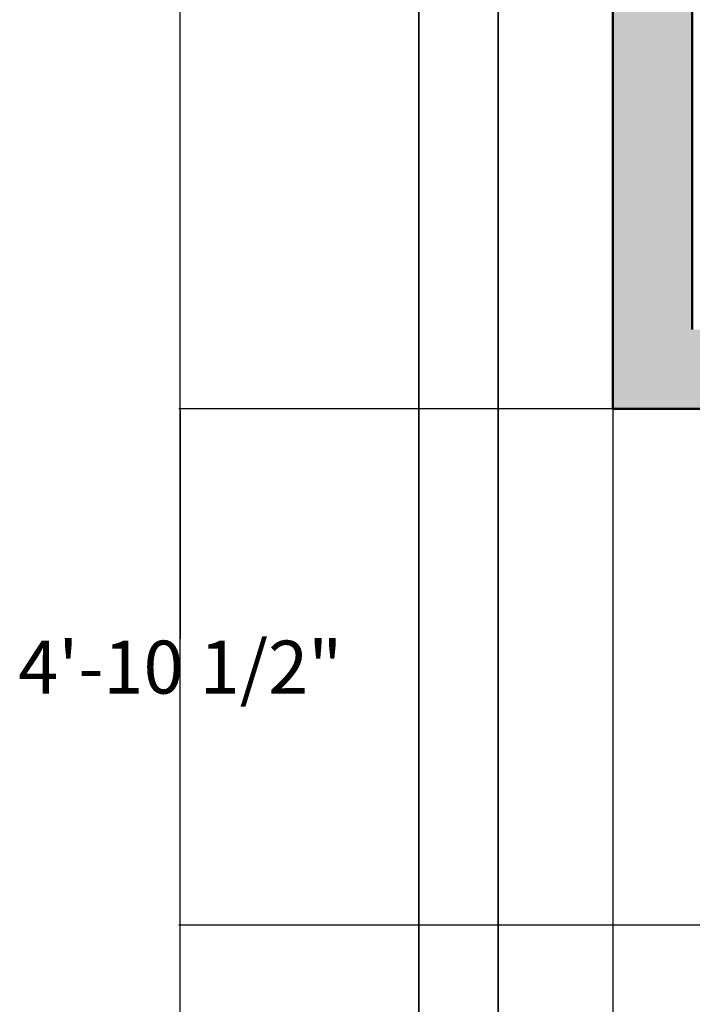
# Model space of a CAD drawing. Units: inches. Extents: x 3398 to 3816, y 15195 to 15771.
# Tile 2 of 10: x 3398 to 3474, y 15306 to 15418. Entities that reach past the tile are written whole.
import ezdxf

# ---------------------------------------------------------------- set-up
doc = ezdxf.new("R2010")
doc.units = ezdxf.units.IN
doc.header["$MEASUREMENT"] = 0
for name, color, linetype, lineweight in [('A-ANNO-DIMS', 2, 'Continuous', 18), ('A-WALL', 7, 'Continuous', 50), ('A-WALL-PATT', 252, 'Continuous', 13), ('C-PROP', 7, 'Continuous', 35)]:
    doc.layers.add(name, color=color, linetype=linetype, lineweight=lineweight)
doc.styles.get("Standard").update_dxf_attribs({"font": 'arial.ttf'})
doc.dimstyles.get("Standard").update_dxf_attribs({"dimtxt": 6, "dimasz": 0.18, "dimexe": 0.18, "dimexo": 0.0625, "dimgap": 0.09, "dimtad": 0, "dimtih": 1, "dimtoh": 1, "dimdec": 1, "dimzin": 0, "dimdsep": 46, "dimlunit": 3, "dimtxsty": 'Standard', "dimcen": 0.09, "dimadec": 0, "dimazin": 0, "dimtfac": 1, "dimtdec": 1, "dimtofl": 0, "dimtmove": 0, "dimatfit": 3, "dimfxl": 1, "dimtolj": 1, "dimtzin": 0, "dimarcsym": 0})

# ---------------------------------------------------------------- blocks, each defined once
blk = doc.blocks.new('*D38')
at = {"layer": 'A-ANNO-DIMS', "color": 0, "lineweight": -2, "transparency": 16777216}
for p, q in [((3465.13, 15730.52), (3415.96, 15730.52)), ((3416.14, 15730.34), (3416.14, 15483.67)), ((3416.14, 15230.7), (3416.14, 15477.37)), ((3465.74, 15230.52), (3415.96, 15230.52))]:
    blk.add_line(p, q, dxfattribs=at)
at = {"layer": 'A-ANNO-DIMS', "color": 0, "transparency": 16777216}
for points in [[(3416.11, 15730.34), (3416.17, 15730.34), (3416.14, 15730.52)], [(3416.11, 15230.7), (3416.17, 15230.7), (3416.14, 15230.52)]]:
    blk.add_solid(points, dxfattribs=at)
at = {"layer": 'Defpoints', "color": 0, "transparency": 16777216}
for p in [(3416.14, 15730.52), (3465.19, 15730.52), (3465.8, 15230.52)]:
    blk.add_point(p, dxfattribs=at)
at = {"layer": 'A-ANNO-DIMS', "color": 0, "transparency": 16777216, "insert": (3416.14, 15480.52), "char_height": 6, "attachment_point": 5}
blk.add_mtext('\\A1;41\'-8"', dxfattribs=at)
blk = doc.blocks.new('*D39')
at = {"layer": 'A-ANNO-DIMS', "color": 0, "lineweight": -2, "transparency": 16777216}
for p, q in [((3465.19, 15373.46), (3465.19, 15203.29)), ((3606.19, 15373.46), (3606.19, 15203.29)), ((3465.37, 15203.47), (3525.58, 15203.47)), ((3606.01, 15203.47), (3545.8, 15203.47))]:
    blk.add_line(p, q, dxfattribs=at)
at = {"layer": 'A-ANNO-DIMS', "color": 0, "transparency": 16777216}
for points in [[(3465.37, 15203.5), (3465.37, 15203.44), (3465.19, 15203.47)], [(3606.01, 15203.5), (3606.01, 15203.44), (3606.19, 15203.47)]]:
    blk.add_solid(points, dxfattribs=at)
at = {"layer": 'Defpoints', "color": 0, "transparency": 16777216}
for p in [(3465.19, 15373.52), (3606.19, 15373.52), (3606.19, 15203.47)]:
    blk.add_point(p, dxfattribs=at)
at = {"layer": 'A-ANNO-DIMS', "color": 0, "transparency": 16777216, "insert": (3535.69, 15203.47), "char_height": 6, "attachment_point": 5}
blk.add_mtext('\\A1;11\'-9"', dxfattribs=at)
blk = doc.blocks.new('*D40')
at = {"layer": 'A-ANNO-DIMS', "color": 0, "lineweight": -2, "transparency": 16777216}
for p, q in [((3465.13, 15373.52), (3415.96, 15373.52)), ((3416.14, 15373.34), (3416.14, 15347.46)), ((3416.14, 15315.2), (3416.14, 15341.08)), ((3606.13, 15315.02), (3415.96, 15315.02))]:
    blk.add_line(p, q, dxfattribs=at)
at = {"layer": 'A-ANNO-DIMS', "color": 0, "transparency": 16777216}
for points in [[(3416.11, 15373.34), (3416.17, 15373.34), (3416.14, 15373.52)], [(3416.11, 15315.2), (3416.17, 15315.2), (3416.14, 15315.02)]]:
    blk.add_solid(points, dxfattribs=at)
at = {"layer": 'Defpoints', "color": 0, "transparency": 16777216}
for p in [(3416.14, 15373.52), (3465.19, 15373.52), (3606.19, 15315.02)]:
    blk.add_point(p, dxfattribs=at)
at = {"layer": 'A-ANNO-DIMS', "color": 0, "transparency": 16777216, "insert": (3416.14, 15344.27), "char_height": 6, "attachment_point": 5}
blk.add_mtext('\\A1;4\'-10 1/2"', dxfattribs=at)

msp = doc.modelspace()

# ---------------------------------------------------------------- hatches: boundary and pattern name
at = {"layer": 'A-WALL-PATT'}
h = msp.add_hatch(color=256, dxfattribs=at)
h.dxf.hatch_style = 1
h.paths.add_polyline_path([(3515.96, 15730.52), (3465.19, 15730.52), (3465.19, 15715.52), (3474.19, 15715.52), (3474.19, 15721.52), (3515.96, 15721.52)])
h.paths.add_polyline_path([(3719.81, 15730.52), (3675.76, 15730.52), (3675.76, 15721.52), (3700.69, 15721.52), (3700.69, 15637.52), (3610.69, 15637.52), (3610.69, 15663.97), (3606.19, 15663.97), (3606.19, 15601.52), (3599.08, 15601.52), (3599.08, 15592.52), (3606.19, 15592.52), (3606.19, 15508.52), (3616.69, 15508.52), (3616.69, 15513.02), (3610.69, 15513.02), (3610.69, 15633.02), (3708.19, 15633.02), (3708.19, 15637.52), (3705.19, 15637.52), (3705.19, 15721.52), (3719.81, 15721.52)])
h.paths.add_polyline_path([(3762.19, 15730.52), (3743.77, 15730.52), (3743.77, 15721.52), (3753.19, 15721.52), (3753.19, 15637.52), (3732.19, 15637.52), (3732.19, 15633.02), (3753.19, 15633.02), (3753.19, 15597.39), (3762.19, 15597.39)])
h.paths.add_polyline_path([(3762.19, 15549.39), (3753.19, 15549.39), (3753.19, 15513.02), (3652.69, 15513.02), (3652.69, 15508.52), (3664.69, 15508.52), (3664.69, 15460.52), (3652.69, 15460.52), (3652.69, 15456.02), (3672.19, 15456.02), (3672.19, 15460.52), (3669.19, 15460.52), (3669.19, 15508.52), (3753.19, 15508.52), (3753.19, 15497.51), (3762.19, 15497.51)])
h.paths.add_polyline_path([(3762.19, 15473.48), (3753.19, 15473.48), (3753.19, 15460.52), (3696.19, 15460.52), (3696.19, 15456.02), (3753.19, 15456.02), (3753.19, 15414.25), (3762.19, 15414.25)])
h.paths.add_polyline_path([(3762.19, 15366.28), (3753.19, 15366.28), (3753.19, 15324.02), (3610.69, 15324.02), (3610.69, 15456.02), (3616.69, 15456.02), (3616.69, 15460.52), (3610.69, 15460.52), (3606.19, 15460.52), (3606.19, 15382.52), (3587.73, 15382.52), (3587.73, 15373.52), (3606.19, 15373.52), (3606.19, 15315.02), (3762.19, 15315.02)])
h.paths.add_polyline_path([(3539.73, 15382.52), (3522.19, 15382.52), (3522.19, 15373.52), (3539.73, 15373.52)])
h.paths.add_polyline_path([(3480.19, 15382.52), (3474.19, 15382.52), (3474.19, 15452.47), (3465.19, 15452.47), (3465.19, 15373.52), (3480.19, 15373.52)])
h.paths.add_polyline_path([(3551.04, 15601.52), (3474.19, 15601.52), (3474.19, 15679.52), (3465.19, 15679.52), (3465.19, 15500.47), (3474.19, 15500.47), (3474.19, 15592.52), (3551.04, 15592.52)])

# ---------------------------------------------------------------- linework, layer by layer
at = {"layer": 'A-WALL'}
for p, q in [((3465.19, 15730.52), (3465.19, 15373.52)), ((3474.19, 15592.52), (3474.19, 15382.52)), ((3465.19, 15373.52), (3606.19, 15373.52))]:
    msp.add_line(p, q, dxfattribs=at)
at = {"layer": 'C-PROP'}
for p, q in [((3443.19, 15739.52), (3443.19, 15230.52)), ((3452.19, 15730.52), (3452.19, 15239.52))]:
    msp.add_line(p, q, dxfattribs=at)

# ---------------------------------------------------------------- dimensions: what is measured, and where the dimension line sits
at = {"layer": 'A-ANNO-DIMS'}
for base, p1, p2, picture, middle in [((3416.14, 15730.52), (3465.8, 15230.52), (3465.19, 15730.52), '*D38', (3416.14, 15480.52)), ((3416.14, 15373.52), (3606.19, 15315.02), (3465.19, 15373.52), '*D40', (3416.14, 15344.27))]:
    dim = msp.add_linear_dim(base=base, p1=p1, p2=p2, angle=90, dimstyle='Standard', override={"dimdec": 1, "dimlfac": 1, "dimrnd": 0, "dimzin": 1, "dimdsep": 46, "dimlunit": 4, "dimfrac": 2}, dxfattribs=at)
    dim.commit()
    dim.dimension.update_dxf_attribs({"geometry": picture, "text_midpoint": middle})
dim = msp.add_linear_dim(base=(3606.19, 15203.47), p1=(3465.19, 15373.52), p2=(3606.19, 15373.52), dimstyle='Standard', override={"dimdec": 1, "dimlfac": 1, "dimrnd": 0, "dimzin": 1, "dimdsep": 46, "dimlunit": 4, "dimfrac": 2}, dxfattribs=at)
dim.commit()
dim.dimension.update_dxf_attribs({"geometry": '*D39', "text_midpoint": (3535.69, 15203.47)})

doc.saveas('drawing.dxf')
